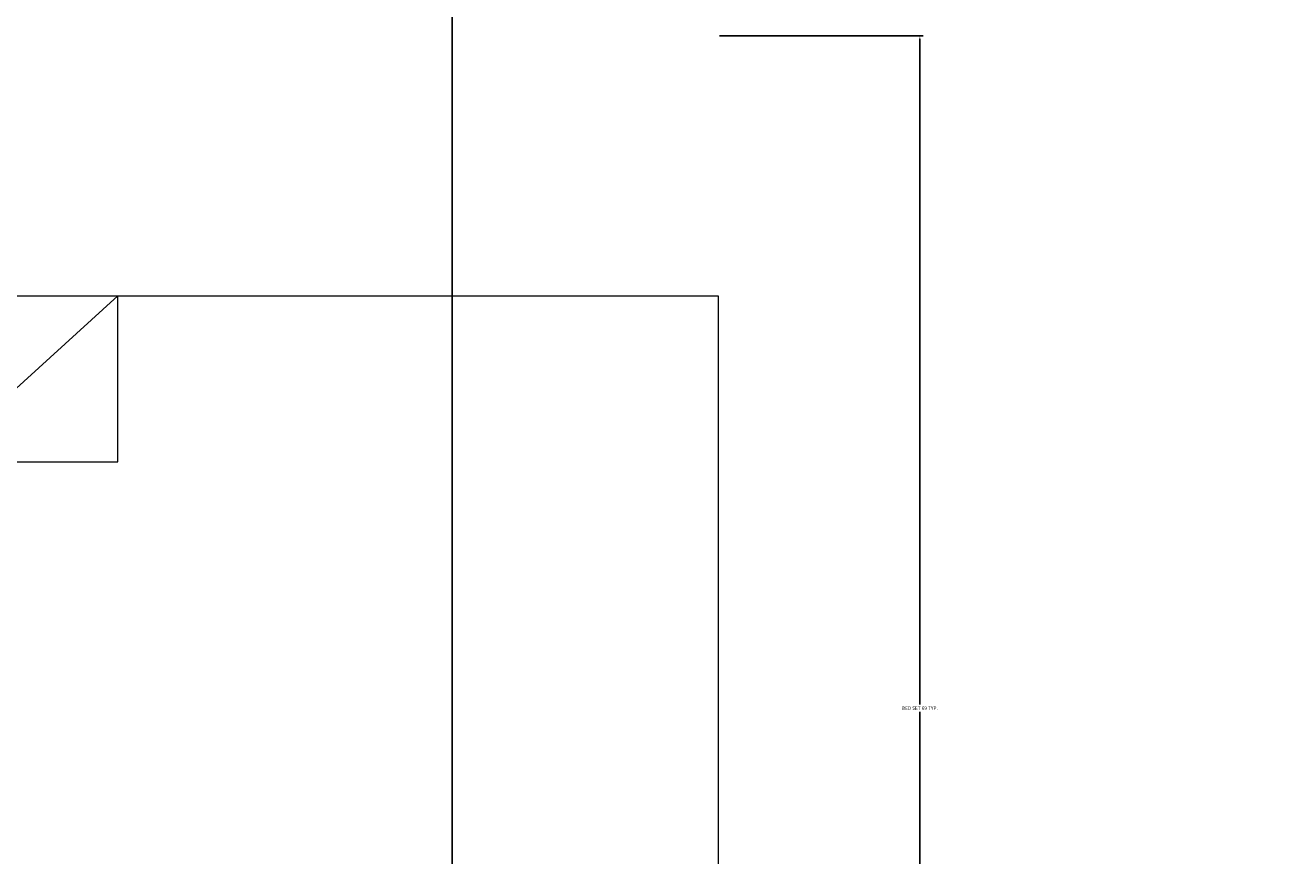
# Model space of a CAD drawing. Units: inches. Extents: x 1998 to 2588, y 1139 to 1977.
# Tile 73 of 134: x 2126 to 2192, y 1817 to 1860. Entities that reach past the tile are written whole.
import ezdxf

# ---------------------------------------------------------------- set-up
doc = ezdxf.new("R2010")
doc.units = ezdxf.units.IN
doc.layers.add('A-ANNO-DIMS', color=2, linetype='Continuous', lineweight=18)
doc.layers.add('FUR', color=21, linetype='Continuous', lineweight=18)
doc.styles.get("Standard").update_dxf_attribs({"font": 'arial.ttf'})
doc.dimstyles.get("Standard").update_dxf_attribs({"dimtxt": 0.18, "dimasz": 0.18, "dimexe": 0.18, "dimexo": 0.0625, "dimgap": 0.09, "dimtad": 0, "dimtih": 1, "dimtoh": 1, "dimdec": 4, "dimzin": 0, "dimdsep": 46, "dimtxsty": 'Standard', "dimcen": 0.09, "dimadec": 0, "dimazin": 0, "dimtfac": 1, "dimtdec": 4, "dimtofl": 0, "dimtmove": 0, "dimatfit": 3, "dimfxl": 1, "dimtolj": 1, "dimtzin": 0, "dimarcsym": 0})

# ---------------------------------------------------------------- blocks, each defined once
blk = doc.blocks.new('BED-WITH-NIGHTSTANDS')
for p, q in [((34.217, 56), (24.799, 47.436)), ((34.217, 47.436), (34.217, 56)), ((24.799, 13.424), (24.799, 47.436)), ((24.799, 47.436), (34.217, 47.436))]:
    blk.add_line(p, q)
for points in [[(0, 56), (15.699, 56), (15.699, 69.425), (0, 69.425)], [(0, 56), (65.221, 56), (65.221, 13.424), (0, 13.424)], [(6.374, 34.93), (16.725, 34.93), (16.725, 53.45), (6.374, 53.45)], [(6.254, 16.049), (16.605, 16.049), (16.605, 34.569), (6.254, 34.569)], [(0, 0), (15.699, 0), (15.699, 13.424), (0, 13.424)]]:
    blk.add_lwpolyline(points, close=True)
blk = doc.blocks.new('*D13')
at = {"layer": 'A-ANNO-DIMS', "color": 0, "lineweight": -2, "transparency": 16777216}
for p, q in [((2162.257, 1859.47), (2172.788, 1859.47)), ((2172.608, 1859.29), (2172.608, 1824.94)), ((2172.608, 1790.225), (2172.608, 1824.574)), ((2162.257, 1790.045), (2172.788, 1790.045))]:
    blk.add_line(p, q, dxfattribs=at)
at = {"layer": 'A-ANNO-DIMS', "color": 0, "transparency": 16777216}
for points in [[(2172.578, 1859.29), (2172.638, 1859.29), (2172.608, 1859.47)], [(2172.578, 1790.225), (2172.638, 1790.225), (2172.608, 1790.045)]]:
    blk.add_solid(points, dxfattribs=at)
at = {"layer": 'Defpoints', "color": 0, "transparency": 16777216}
for p in [(2162.194, 1859.47), (2172.608, 1859.47), (2162.194, 1790.045)]:
    blk.add_point(p, dxfattribs=at)
at = {"layer": 'A-ANNO-DIMS', "color": 0, "transparency": 16777216, "insert": (2172.608, 1824.757), "char_height": 0.18, "attachment_point": 5}
blk.add_mtext('\\A1;BED SET 69 TYP.', dxfattribs=at)
blk = doc.blocks.new('*D37')
at = {"layer": 'A-ANNO-DIMS', "color": 0, "lineweight": -2, "transparency": 16777216}
for p, q in [((2148.455, 1612.795), (2148.455, 1977.362)), ((2148.635, 1977.182), (2172.73, 1977.182)), ((2197.27, 1977.182), (2173.175, 1977.182)), ((2197.45, 1612.795), (2197.45, 1977.362))]:
    blk.add_line(p, q, dxfattribs=at)
at = {"layer": 'A-ANNO-DIMS', "color": 0, "transparency": 16777216}
for points in [[(2148.635, 1977.212), (2148.635, 1977.152), (2148.455, 1977.182)], [(2197.27, 1977.212), (2197.27, 1977.152), (2197.45, 1977.182)]]:
    blk.add_solid(points, dxfattribs=at)
at = {"layer": 'Defpoints', "color": 0, "transparency": 16777216}
for p in [(2197.45, 1977.182), (2148.455, 1612.732), (2197.45, 1612.732)]:
    blk.add_point(p, dxfattribs=at)
at = {"layer": 'A-ANNO-DIMS', "color": 0, "transparency": 16777216, "insert": (2172.952, 1977.182), "char_height": 0.18, "attachment_point": 5}
blk.add_mtext('\\A1;49', dxfattribs=at)

msp = doc.modelspace()

# ---------------------------------------------------------------- block references
at = {"layer": 'FUR'}
msp.add_blockref('BED-WITH-NIGHTSTANDS', (2096.973, 1790.045), dxfattribs=at)

# ---------------------------------------------------------------- dimensions: what is measured, and where the dimension line sits
at = {"layer": 'A-ANNO-DIMS'}
dim = msp.add_linear_dim(base=(2197.4499, 1977.1824), p1=(2148.4548, 1612.7324), p2=(2197.4499, 1612.7324), dimstyle='Standard', override={"dimdec": 0, "dimlfac": 1, "dimrnd": 0, "dimzin": 0, "dimdsep": 46, "dimlunit": 2}, dxfattribs=at)
dim.commit()
dim.dimension.update_dxf_attribs({"geometry": '*D37', "text_midpoint": (2172.9524, 1977.1824)})
dim = msp.add_linear_dim(base=(2172.6081, 1859.4697), p1=(2162.1944, 1790.0445), p2=(2162.1944, 1859.4697), angle=90, text='BED SET <> TYP.', dimstyle='Standard', override={"dimdec": 0, "dimlfac": 1, "dimrnd": 0, "dimzin": 0, "dimdsep": 46, "dimlunit": 2}, dxfattribs=at)
dim.commit()
dim.dimension.update_dxf_attribs({"geometry": '*D13', "text_midpoint": (2172.6081, 1824.7571)})

doc.saveas('drawing.dxf')
